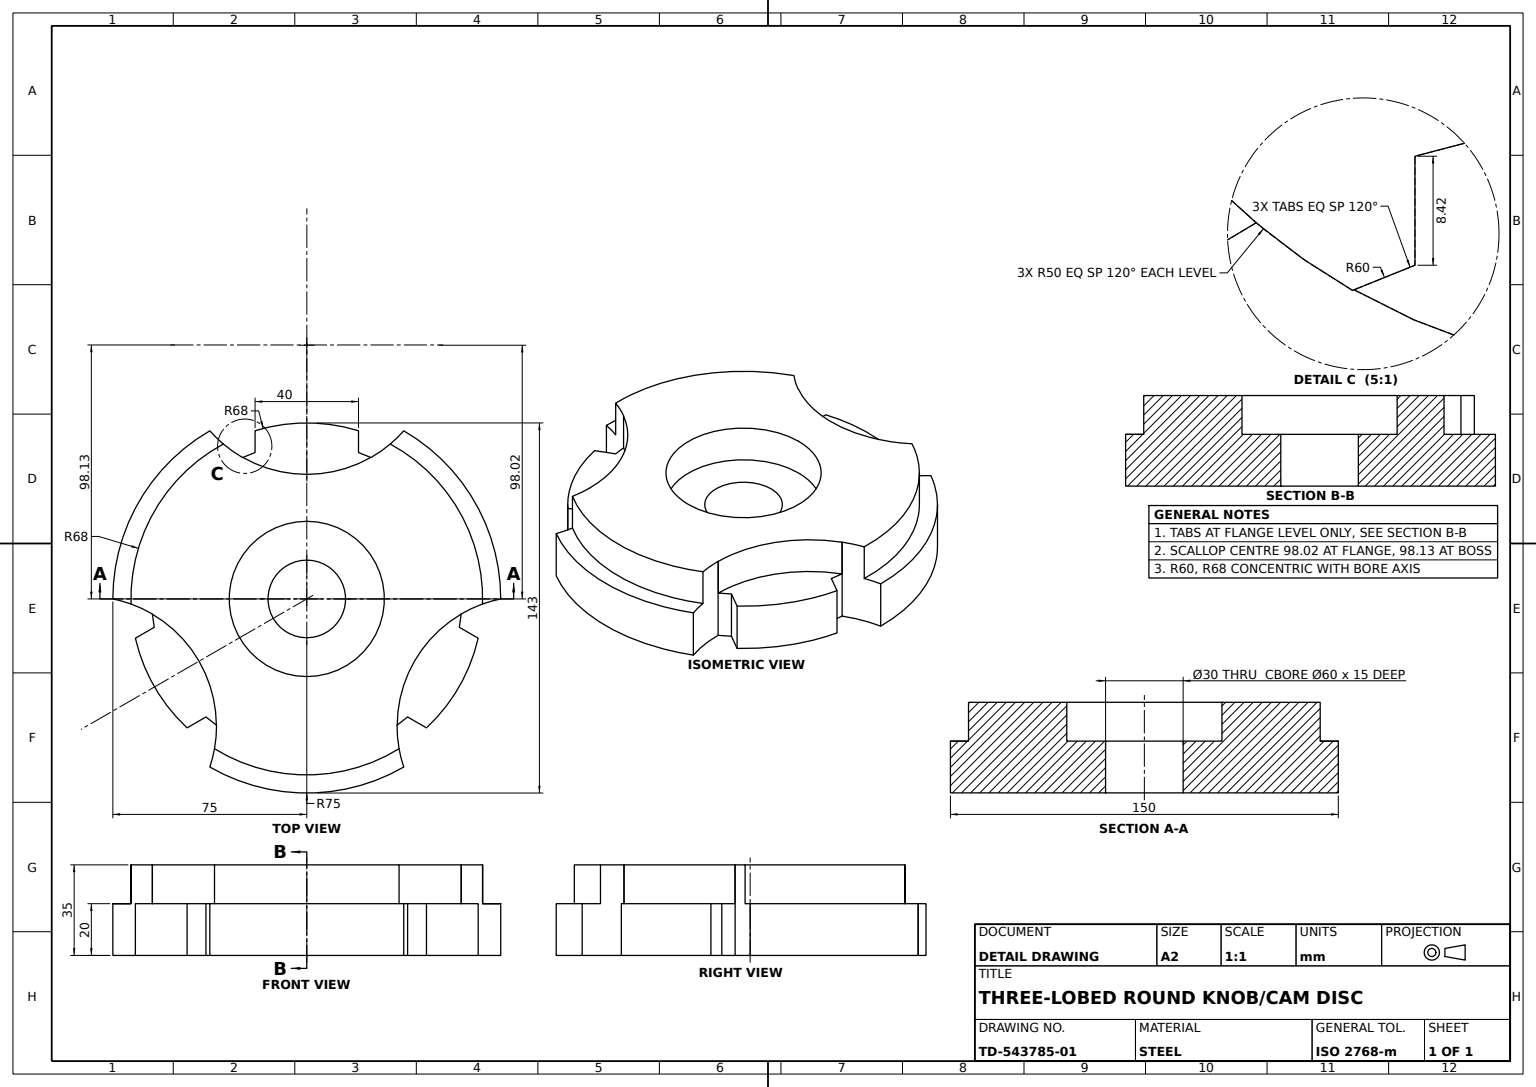
SolidWorks part; units mm, degrees
material "Plain Carbon Steel"
ref_plane "Front Plane" through (0, 0, 0) normal (0, 0, 1) x (1, 0, 0)
ref_plane "Top Plane" through (0, 0, 0) normal (0, 1, 0) x (1, 0, 0)
ref_plane "Right Plane" through (0, 0, 0) normal (1, 0, 0) x (0, 0, -1)
sketch "Lobed Base Profile" plane through (0, 0, 0) normal (0, 1, 0) x (1, 0, 0)
  arc A0 (-37.5, 64.9519) -> (-75, 0) centre (0, 0) ccw
  arc A1 (75, 0) -> (37.5, 64.9519) centre (0, 0) ccw
  arc A2 (-37.5, -64.9519) -> (37.5, -64.9519) centre (0, 0) ccw
  arc A3 (-75, 0) -> (-37.5, -64.9519) centre (-84.8911, -49.0119) cw
  arc A4 (37.5, 64.9519) -> (-37.5, 64.9519) centre (0, 98.0238) cw
  arc A5 (37.5, -64.9519) -> (75, 0) centre (84.8911, -49.0119) cw
  dimension "D1" = 50
  dimension "D2" = 75
  dimension "D5" = 3
  dimension "D3" = 37.5
  dimension "D4" = 64.9519
extrude "Lobed Base 20mm" add sketch "Lobed Base Profile" along normal blind 20
sketch "Notched Step Profile" plane through (0, 20, 0) normal (0, 1, 0) x (1, 0, 0)
  line L0 (66.285, -15.1756) -> (58.9898, -10.9638)
  line L1 (20, 64.9923) -> (20, 56.5685)
  line L2 (46.285, -49.8167) -> (38.9898, -45.6048)
  line L3 (-20, 64.9923) -> (-20, 56.5685)
  line L4 (-46.285, -49.8167) -> (-38.9898, -45.6048)
  line L5 (-66.285, -15.1756) -> (-58.9898, -10.9638)
  arc A0 (20, 64.9923) -> (-20, 64.9923) centre (0, 0) ccw
  arc A1 (-20, 56.5685) -> (-24.8264, 54.6228) centre (0, 0) ccw
  arc A2 (-24.8264, 54.6228) -> (24.8264, 54.6228) centre (0, 98.0238) ccw
  arc A3 (24.8264, 54.6228) -> (20, 56.5685) centre (0, 0) ccw
  arc A4 (46.285, -49.8167) -> (66.285, -15.1756) centre (0, 0) ccw
  arc A5 (34.8915, -48.8117) -> (38.9898, -45.6048) centre (0, 0) ccw
  arc A6 (59.7179, -5.8111) -> (34.8915, -48.8117) centre (84.8911, -49.0119) ccw
  arc A7 (58.9898, -10.9638) -> (59.7179, -5.8111) centre (0, 0) ccw
  arc A8 (-66.285, -15.1756) -> (-46.285, -49.8167) centre (0, 0) ccw
  arc A9 (-59.7179, -5.8111) -> (-58.9898, -10.9638) centre (0, 0) ccw
  arc A10 (-34.8915, -48.8117) -> (-59.7179, -5.8111) centre (-84.8911, -49.0119) ccw
  arc A11 (-38.9898, -45.6048) -> (-34.8915, -48.8117) centre (0, 0) ccw
  dimension "D1" = 3
  dimension "D2" = 68
  dimension "D3" = 50
  dimension "D6" = 60
  dimension "D4" = 49.0119
  dimension "D5" = 84.8911
  dimension "D7" = 8.4238
  dimension "D8" = 8.4238
extrude "Notched Step Boss 20mm" add sketch "Notched Step Profile" against normal blind 20
sketch "Lobed Top Step Profile" plane through (0, 20, 0) normal (0, 1, 0) x (1, 0, 0)
  arc A0 (-35.7438, -57.8479) -> (35.7438, -57.8479) centre (0, 0) ccw
  arc A1 (-34, -58.8897) -> (34, -58.8897) centre (0, 0) ccw
  arc A2 (67.9708, -1.9938) -> (32.2258, 59.879) centre (0, 0) ccw
  arc A6 (-32.1982, 59.8938) -> (32.2258, 59.879) centre (0.0226, 98.1276) ccw
  arc A7 (67.9708, -1.9938) -> (35.7438, -57.8479) centre (84.9583, -49.0196) ccw
  arc A10 (-32.1982, 59.8938) -> (-67.9697, -2.0311) centre (0, 0) ccw
  arc A11 (68, 0) -> (32.2258, 59.879) centre (0, 0) ccw
  arc A13 (-67.9697, -2.0311) -> (-35.7438, -57.8479) centre (-84.9645, -49.0543) cw
  arc M1 (-75, 0) -> (-59.7179, -5.8111) centre (-84.8911, -49.0119) cw
  arc M2 (-59.7179, -5.8111) -> (-58.9898, -10.9638) centre (0, 0) ccw
  arc M6 (-38.9898, -45.6048) -> (-34.8915, -48.8117) centre (0, 0) ccw
  arc M7 (-34.8915, -48.8117) -> (-37.5, -64.9519) centre (-84.8911, -49.0119) cw
  arc M9 (37.5, -64.9519) -> (34.8915, -48.8117) centre (84.8911, -49.0119) cw
  arc M10 (34.8915, -48.8117) -> (38.9898, -45.6048) centre (0, 0) ccw
  arc M14 (58.9898, -10.9638) -> (59.7179, -5.8111) centre (0, 0) ccw
  arc M15 (59.7179, -5.8111) -> (75, 0) centre (84.8911, -49.0119) cw
  arc M17 (37.5, 64.9519) -> (24.8264, 54.6228) centre (0, 98.0238) cw
  arc M18 (24.8264, 54.6228) -> (20, 56.5685) centre (0, 0) ccw
  arc M22 (-20, 56.5685) -> (-24.8264, 54.6228) centre (0, 0) ccw
  arc M23 (-24.8264, 54.6228) -> (-37.5, 64.9519) centre (0, 98.0238) cw
  dimension "D1" = 3
  dimension "D2" = 68
  dimension "D6" = 35.7438
  dimension "D7" = 57.8479
  dimension "D8" = 50
  dimension "D9" = 50
  dimension "D10" = 50
  dimension "D3" = 3
  dimension "D4" = 58.8897
  dimension "D5" = 34
  dimension "D11" = 49.0196
  dimension "D12" = 84.9645
  dimension "D13" = 84.9357
  dimension "D14" = 147.1819
extrude "Lobed Top Step Boss 15mm" add sketch "Lobed Top Step Profile" along normal blind 15 contours A13 A0 A7 A2 A6 A10 M2 M6 M7 M9 M10 M14 M15 M17 M18 M22 M23 M1
sketch "Counterbore Profile Ø60" plane through (0, 35, 0) normal (0, 1, 0) x (1, 0, 0)
  circle A0 centre (0, 0) radius 30
  dimension "D1" = 60
extrude "Counterbore Ø60x15" cut sketch "Counterbore Profile Ø60" against normal blind 15
sketch "Center Bore Profile Ø30" plane through (0, 20, 0) normal (0, 1, 0) x (1, 0, 0)
  circle A0 centre (0, 0) radius 15
  dimension "D1" = 30
extrude "Center Bore Ø30" cut sketch "Center Bore Profile Ø30" against normal blind 60
